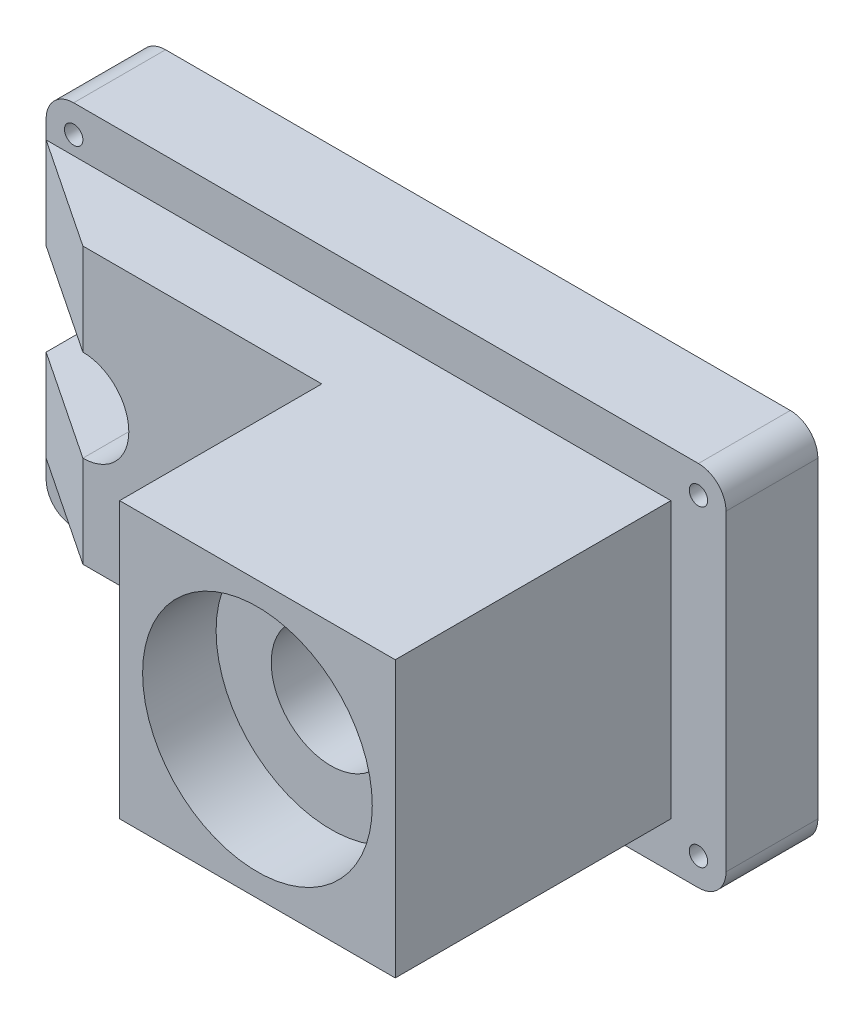
ISO-10303-21;
HEADER;
FILE_DESCRIPTION(('STEP AP214'),'2;1');
FILE_NAME('part.step','',(''),(''),'','','');
FILE_SCHEMA(('AUTOMOTIVE_DESIGN { 1 0 10303 214 1 1 1 1 }'));
ENDSEC;
DATA;
#1=APPLICATION_CONTEXT('core data for automotive mechanical design processes');
#2=APPLICATION_PROTOCOL_DEFINITION('international standard','automotive_design',2000,#1);
#3=PRODUCT_CONTEXT('',#1,'mechanical');
#4=PRODUCT('Part','Part','',(#3));
#5=PRODUCT_RELATED_PRODUCT_CATEGORY('part','',(#4));
#6=PRODUCT_DEFINITION_FORMATION('','',#4);
#7=PRODUCT_DEFINITION_CONTEXT('part definition',#1,'design');
#8=PRODUCT_DEFINITION('design','',#6,#7);
#9=PRODUCT_DEFINITION_SHAPE('','',#8);
#10=(LENGTH_UNIT() NAMED_UNIT(*) SI_UNIT(.MILLI.,.METRE.));
#11=(NAMED_UNIT(*) PLANE_ANGLE_UNIT() SI_UNIT($,.RADIAN.));
#12=(NAMED_UNIT(*) SI_UNIT($,.STERADIAN.) SOLID_ANGLE_UNIT());
#13=UNCERTAINTY_MEASURE_WITH_UNIT(LENGTH_MEASURE(1.E-05),#10,'distance_accuracy_value','');
#14=(GEOMETRIC_REPRESENTATION_CONTEXT(3) GLOBAL_UNCERTAINTY_ASSIGNED_CONTEXT((#13)) GLOBAL_UNIT_ASSIGNED_CONTEXT((#10,
#11,#12)) REPRESENTATION_CONTEXT('',''));
#15=CARTESIAN_POINT('',(0.,0.,0.));
#16=DIRECTION('',(0.,0.,1.));
#17=DIRECTION('',(1.,0.,0.));
#18=AXIS2_PLACEMENT_3D('',#15,#16,#17);
#19=CARTESIAN_POINT('',(3.,37.,10.));
#20=DIRECTION('',(0.,0.,1.));
#21=DIRECTION('',(1.,0.,0.));
#22=AXIS2_PLACEMENT_3D('',#19,#20,#21);
#23=PLANE('',#22);
#24=CARTESIAN_POINT('',(3.,3.,10.));
#25=DIRECTION('',(0.,0.,1.));
#26=DIRECTION('',(1.,0.,0.));
#27=AXIS2_PLACEMENT_3D('',#24,#25,#26);
#28=CIRCLE('',#27,1.);
#29=CARTESIAN_POINT('',(4.,3.,10.));
#30=VERTEX_POINT('',#29);
#31=EDGE_CURVE('E352',#30,#30,#28,.T.);
#32=ORIENTED_EDGE('',*,*,#31,.F.);
#33=EDGE_LOOP('',(#32));
#34=FACE_BOUND('',#33,.T.);
#35=CARTESIAN_POINT('',(71.,3.,10.));
#36=DIRECTION('',(0.,0.,1.));
#37=DIRECTION('',(1.,0.,0.));
#38=AXIS2_PLACEMENT_3D('',#35,#36,#37);
#39=CIRCLE('',#38,0.999999999999998);
#40=CARTESIAN_POINT('',(72.,3.,10.));
#41=VERTEX_POINT('',#40);
#42=EDGE_CURVE('E356',#41,#41,#39,.T.);
#43=ORIENTED_EDGE('',*,*,#42,.F.);
#44=EDGE_LOOP('',(#43));
#45=FACE_BOUND('',#44,.T.);
#46=CARTESIAN_POINT('',(71.,37.,10.));
#47=DIRECTION('',(0.,0.,1.));
#48=DIRECTION('',(1.,0.,0.));
#49=AXIS2_PLACEMENT_3D('',#46,#47,#48);
#50=CIRCLE('',#49,0.999999999999998);
#51=CARTESIAN_POINT('',(72.,37.,10.));
#52=VERTEX_POINT('',#51);
#53=EDGE_CURVE('E364',#52,#52,#50,.T.);
#54=ORIENTED_EDGE('',*,*,#53,.F.);
#55=EDGE_LOOP('',(#54));
#56=FACE_BOUND('',#55,.T.);
#57=CARTESIAN_POINT('',(3.,37.,10.));
#58=DIRECTION('',(0.,0.,1.));
#59=DIRECTION('',(1.,0.,0.));
#60=AXIS2_PLACEMENT_3D('',#57,#58,#59);
#61=CIRCLE('',#60,0.999999999999998);
#62=CARTESIAN_POINT('',(4.,37.,10.));
#63=VERTEX_POINT('',#62);
#64=EDGE_CURVE('E342',#63,#63,#61,.T.);
#65=ORIENTED_EDGE('',*,*,#64,.F.);
#66=EDGE_LOOP('',(#65));
#67=FACE_BOUND('',#66,.T.);
#68=DIRECTION('',(0.,-1.,0.));
#69=VECTOR('',#68,1.);
#70=CARTESIAN_POINT('',(0.,37.,10.));
#71=LINE('',#70,#69);
#72=CARTESIAN_POINT('',(0.,37.,10.));
#73=VERTEX_POINT('',#72);
#74=CARTESIAN_POINT('',(0.,35.,10.));
#75=VERTEX_POINT('',#74);
#76=EDGE_CURVE('E247',#73,#75,#71,.T.);
#77=ORIENTED_EDGE('',*,*,#76,.T.);
#78=DIRECTION('',(-1.,0.,0.));
#79=VECTOR('',#78,1.);
#80=CARTESIAN_POINT('',(68.,35.,10.));
#81=LINE('',#80,#79);
#82=CARTESIAN_POINT('',(68.,35.,10.));
#83=VERTEX_POINT('',#82);
#84=EDGE_CURVE('E58',#83,#75,#81,.T.);
#85=ORIENTED_EDGE('',*,*,#84,.F.);
#86=DIRECTION('',(0.,1.,0.));
#87=VECTOR('',#86,1.);
#88=CARTESIAN_POINT('',(68.,35.,10.));
#89=LINE('',#88,#87);
#90=CARTESIAN_POINT('',(68.,4.99999999999999,10.));
#91=VERTEX_POINT('',#90);
#92=EDGE_CURVE('E216',#91,#83,#89,.T.);
#93=ORIENTED_EDGE('',*,*,#92,.F.);
#94=DIRECTION('',(1.,0.,0.));
#95=VECTOR('',#94,1.);
#96=CARTESIAN_POINT('',(68.,4.99999999999999,10.));
#97=LINE('',#96,#95);
#98=CARTESIAN_POINT('',(0.,4.99999999999998,10.));
#99=VERTEX_POINT('',#98);
#100=EDGE_CURVE('E69',#99,#91,#97,.T.);
#101=ORIENTED_EDGE('',*,*,#100,.F.);
#102=DIRECTION('',(0.,-1.,0.));
#103=VECTOR('',#102,1.);
#104=CARTESIAN_POINT('',(0.,15.,10.));
#105=LINE('',#104,#103);
#106=CARTESIAN_POINT('',(0.,3.,10.));
#107=VERTEX_POINT('',#106);
#108=EDGE_CURVE('E255',#99,#107,#105,.T.);
#109=ORIENTED_EDGE('',*,*,#108,.T.);
#110=CARTESIAN_POINT('',(3.,3.,10.));
#111=DIRECTION('',(0.,0.,1.));
#112=DIRECTION('',(1.,0.,0.));
#113=AXIS2_PLACEMENT_3D('',#110,#111,#112);
#114=CIRCLE('',#113,3.);
#115=CARTESIAN_POINT('',(3.,0.,10.));
#116=VERTEX_POINT('',#115);
#117=EDGE_CURVE('E253',#107,#116,#114,.T.);
#118=ORIENTED_EDGE('',*,*,#117,.T.);
#119=DIRECTION('',(1.,0.,0.));
#120=VECTOR('',#119,1.);
#121=CARTESIAN_POINT('',(3.,0.,10.));
#122=LINE('',#121,#120);
#123=CARTESIAN_POINT('',(71.,0.,10.));
#124=VERTEX_POINT('',#123);
#125=EDGE_CURVE('E256',#116,#124,#122,.T.);
#126=ORIENTED_EDGE('',*,*,#125,.T.);
#127=CARTESIAN_POINT('',(71.,3.,10.));
#128=DIRECTION('',(0.,0.,1.));
#129=DIRECTION('',(1.,0.,0.));
#130=AXIS2_PLACEMENT_3D('',#127,#128,#129);
#131=CIRCLE('',#130,3.);
#132=CARTESIAN_POINT('',(74.,3.,10.));
#133=VERTEX_POINT('',#132);
#134=EDGE_CURVE('E258',#124,#133,#131,.T.);
#135=ORIENTED_EDGE('',*,*,#134,.T.);
#136=DIRECTION('',(0.,1.,0.));
#137=VECTOR('',#136,1.);
#138=CARTESIAN_POINT('',(74.,37.,10.));
#139=LINE('',#138,#137);
#140=CARTESIAN_POINT('',(74.,37.,10.));
#141=VERTEX_POINT('',#140);
#142=EDGE_CURVE('E262',#133,#141,#139,.T.);
#143=ORIENTED_EDGE('',*,*,#142,.T.);
#144=CARTESIAN_POINT('',(71.,37.,10.));
#145=DIRECTION('',(0.,0.,1.));
#146=DIRECTION('',(1.,0.,0.));
#147=AXIS2_PLACEMENT_3D('',#144,#145,#146);
#148=CIRCLE('',#147,3.00000000000001);
#149=CARTESIAN_POINT('',(71.,40.,10.));
#150=VERTEX_POINT('',#149);
#151=EDGE_CURVE('E264',#141,#150,#148,.T.);
#152=ORIENTED_EDGE('',*,*,#151,.T.);
#153=DIRECTION('',(-1.,0.,0.));
#154=VECTOR('',#153,1.);
#155=CARTESIAN_POINT('',(3.,40.,10.));
#156=LINE('',#155,#154);
#157=CARTESIAN_POINT('',(3.,40.,10.));
#158=VERTEX_POINT('',#157);
#159=EDGE_CURVE('E263',#150,#158,#156,.T.);
#160=ORIENTED_EDGE('',*,*,#159,.T.);
#161=CARTESIAN_POINT('',(3.,37.,10.));
#162=DIRECTION('',(0.,0.,1.));
#163=DIRECTION('',(1.,0.,0.));
#164=AXIS2_PLACEMENT_3D('',#161,#162,#163);
#165=CIRCLE('',#164,3.);
#166=EDGE_CURVE('E244',#158,#73,#165,.T.);
#167=ORIENTED_EDGE('',*,*,#166,.T.);
#168=EDGE_LOOP('',(#77,#85,#93,#101,#109,#118,#126,#135,#143,#152,#160,#167));
#169=FACE_BOUND('',#168,.T.);
#170=ADVANCED_FACE('F44',(#34,#45,#56,#67,#169),#23,.T.);
#171=CARTESIAN_POINT('',(38.,35.,40.));
#172=DIRECTION('',(1.,0.,0.));
#173=DIRECTION('',(0.,0.,-1.));
#174=AXIS2_PLACEMENT_3D('',#171,#172,#173);
#175=PLANE('',#174);
#176=DIRECTION('',(0.,1.,0.));
#177=VECTOR('',#176,1.);
#178=CARTESIAN_POINT('',(38.,35.,18.));
#179=LINE('',#178,#177);
#180=CARTESIAN_POINT('',(38.,4.99999999999999,18.));
#181=VERTEX_POINT('',#180);
#182=CARTESIAN_POINT('',(38.,35.,18.));
#183=VERTEX_POINT('',#182);
#184=EDGE_CURVE('E193',#181,#183,#179,.T.);
#185=ORIENTED_EDGE('',*,*,#184,.F.);
#186=DIRECTION('',(0.,0.,-1.));
#187=VECTOR('',#186,1.);
#188=CARTESIAN_POINT('',(38.,4.99999999999999,40.));
#189=LINE('',#188,#187);
#190=CARTESIAN_POINT('',(38.,4.99999999999999,40.));
#191=VERTEX_POINT('',#190);
#192=EDGE_CURVE('E236',#191,#181,#189,.T.);
#193=ORIENTED_EDGE('',*,*,#192,.F.);
#194=DIRECTION('',(0.,-1.,0.));
#195=VECTOR('',#194,1.);
#196=CARTESIAN_POINT('',(38.,35.,40.));
#197=LINE('',#196,#195);
#198=CARTESIAN_POINT('',(38.,35.,40.));
#199=VERTEX_POINT('',#198);
#200=EDGE_CURVE('E223',#199,#191,#197,.T.);
#201=ORIENTED_EDGE('',*,*,#200,.F.);
#202=DIRECTION('',(0.,0.,-1.));
#203=VECTOR('',#202,1.);
#204=CARTESIAN_POINT('',(38.,35.,40.));
#205=LINE('',#204,#203);
#206=EDGE_CURVE('E237',#199,#183,#205,.T.);
#207=ORIENTED_EDGE('',*,*,#206,.T.);
#208=EDGE_LOOP('',(#185,#193,#201,#207));
#209=FACE_BOUND('',#208,.T.);
#210=ADVANCED_FACE('F331',(#209),#175,.F.);
#211=CARTESIAN_POINT('',(3.,37.,10.));
#212=DIRECTION('',(0.,0.,-1.));
#213=DIRECTION('',(-1.,0.,0.));
#214=AXIS2_PLACEMENT_3D('',#211,#212,#213);
#215=CYLINDRICAL_SURFACE('',#214,3.);
#216=CARTESIAN_POINT('',(3.,37.,0.));
#217=DIRECTION('',(0.,0.,1.));
#218=DIRECTION('',(1.,0.,0.));
#219=AXIS2_PLACEMENT_3D('',#216,#217,#218);
#220=CIRCLE('',#219,3.);
#221=CARTESIAN_POINT('',(3.,40.,0.));
#222=VERTEX_POINT('',#221);
#223=CARTESIAN_POINT('',(0.,37.,0.));
#224=VERTEX_POINT('',#223);
#225=EDGE_CURVE('E242',#222,#224,#220,.T.);
#226=ORIENTED_EDGE('',*,*,#225,.T.);
#227=DIRECTION('',(0.,0.,-1.));
#228=VECTOR('',#227,1.);
#229=CARTESIAN_POINT('',(0.,37.,10.));
#230=LINE('',#229,#228);
#231=EDGE_CURVE('E11',#73,#224,#230,.T.);
#232=ORIENTED_EDGE('',*,*,#231,.F.);
#233=ORIENTED_EDGE('',*,*,#166,.F.);
#234=DIRECTION('',(0.,0.,-1.));
#235=VECTOR('',#234,1.);
#236=CARTESIAN_POINT('',(3.,40.,10.));
#237=LINE('',#236,#235);
#238=EDGE_CURVE('E270',#158,#222,#237,.T.);
#239=ORIENTED_EDGE('',*,*,#238,.T.);
#240=EDGE_LOOP('',(#226,#232,#233,#239));
#241=FACE_BOUND('',#240,.T.);
#242=ADVANCED_FACE('F50',(#241),#215,.T.);
#243=CARTESIAN_POINT('',(0.,37.,10.));
#244=DIRECTION('',(1.,0.,0.));
#245=DIRECTION('',(0.,0.,-1.));
#246=AXIS2_PLACEMENT_3D('',#243,#244,#245);
#247=PLANE('',#246);
#248=DIRECTION('',(0.,-1.,0.));
#249=VECTOR('',#248,1.);
#250=CARTESIAN_POINT('',(0.,37.,0.));
#251=LINE('',#250,#249);
#252=CARTESIAN_POINT('',(0.,25.,0.));
#253=VERTEX_POINT('',#252);
#254=EDGE_CURVE('E268',#224,#253,#251,.T.);
#255=ORIENTED_EDGE('',*,*,#254,.T.);
#256=DIRECTION('',(0.,0.,-1.));
#257=VECTOR('',#256,1.);
#258=CARTESIAN_POINT('',(0.,25.,10.));
#259=LINE('',#258,#257);
#260=CARTESIAN_POINT('',(0.,25.,10.));
#261=VERTEX_POINT('',#260);
#262=EDGE_CURVE('E52',#261,#253,#259,.T.);
#263=ORIENTED_EDGE('',*,*,#262,.F.);
#264=DIRECTION('',(0.,1.,0.));
#265=VECTOR('',#264,1.);
#266=CARTESIAN_POINT('',(0.,25.,10.));
#267=LINE('',#266,#265);
#268=EDGE_CURVE('E209',#261,#75,#267,.T.);
#269=ORIENTED_EDGE('',*,*,#268,.T.);
#270=ORIENTED_EDGE('',*,*,#76,.F.);
#271=ORIENTED_EDGE('',*,*,#231,.T.);
#272=EDGE_LOOP('',(#255,#263,#269,#270,#271));
#273=FACE_BOUND('',#272,.T.);
#274=ADVANCED_FACE('F415',(#273),#247,.F.);
#275=CARTESIAN_POINT('',(12.,25.,10.));
#276=DIRECTION('',(0.,1.,0.));
#277=DIRECTION('',(0.,0.,1.));
#278=AXIS2_PLACEMENT_3D('',#275,#276,#277);
#279=PLANE('',#278);
#280=DIRECTION('',(1.,0.,0.));
#281=VECTOR('',#280,1.);
#282=CARTESIAN_POINT('',(12.,25.,0.));
#283=LINE('',#282,#281);
#284=CARTESIAN_POINT('',(12.,25.,0.));
#285=VERTEX_POINT('',#284);
#286=EDGE_CURVE('E275',#253,#285,#283,.T.);
#287=ORIENTED_EDGE('',*,*,#286,.T.);
#288=DIRECTION('',(0.,0.,-1.));
#289=VECTOR('',#288,1.);
#290=CARTESIAN_POINT('',(12.,25.,10.));
#291=LINE('',#290,#289);
#292=CARTESIAN_POINT('',(12.,25.,18.));
#293=VERTEX_POINT('',#292);
#294=EDGE_CURVE('E185',#293,#285,#291,.T.);
#295=ORIENTED_EDGE('',*,*,#294,.F.);
#296=DIRECTION('',(0.832050294337844,0.,0.554700196225229));
#297=VECTOR('',#296,1.);
#298=CARTESIAN_POINT('',(0.,25.,10.));
#299=LINE('',#298,#297);
#300=EDGE_CURVE('E317',#261,#293,#299,.T.);
#301=ORIENTED_EDGE('',*,*,#300,.F.);
#302=ORIENTED_EDGE('',*,*,#262,.T.);
#303=EDGE_LOOP('',(#287,#295,#301,#302));
#304=FACE_BOUND('',#303,.T.);
#305=ADVANCED_FACE('F314',(#304),#279,.F.);
#306=CARTESIAN_POINT('',(12.,20.,10.));
#307=DIRECTION('',(0.,0.,-1.));
#308=DIRECTION('',(-1.,0.,0.));
#309=AXIS2_PLACEMENT_3D('',#306,#307,#308);
#310=CYLINDRICAL_SURFACE('',#309,5.);
#311=CARTESIAN_POINT('',(12.,20.,0.));
#312=DIRECTION('',(0.,0.,-1.));
#313=DIRECTION('',(1.,0.,0.));
#314=AXIS2_PLACEMENT_3D('',#311,#312,#313);
#315=CIRCLE('',#314,5.);
#316=CARTESIAN_POINT('',(12.,15.,0.));
#317=VERTEX_POINT('',#316);
#318=EDGE_CURVE('E178',#285,#317,#315,.T.);
#319=ORIENTED_EDGE('',*,*,#318,.T.);
#320=DIRECTION('',(0.,0.,-1.));
#321=VECTOR('',#320,1.);
#322=CARTESIAN_POINT('',(12.,15.,10.));
#323=LINE('',#322,#321);
#324=CARTESIAN_POINT('',(12.,15.,18.));
#325=VERTEX_POINT('',#324);
#326=EDGE_CURVE('E171',#325,#317,#323,.T.);
#327=ORIENTED_EDGE('',*,*,#326,.F.);
#328=CARTESIAN_POINT('',(12.,20.,18.));
#329=DIRECTION('',(0.,0.,-1.));
#330=DIRECTION('',(-1.,0.,0.));
#331=AXIS2_PLACEMENT_3D('',#328,#329,#330);
#332=CIRCLE('',#331,5.);
#333=EDGE_CURVE('E174',#293,#325,#332,.T.);
#334=ORIENTED_EDGE('',*,*,#333,.F.);
#335=ORIENTED_EDGE('',*,*,#294,.T.);
#336=EDGE_LOOP('',(#319,#327,#334,#335));
#337=FACE_BOUND('',#336,.T.);
#338=ADVANCED_FACE('F173',(#337),#310,.F.);
#339=CARTESIAN_POINT('',(12.,15.,10.));
#340=DIRECTION('',(0.,-1.,0.));
#341=DIRECTION('',(0.,0.,-1.));
#342=AXIS2_PLACEMENT_3D('',#339,#340,#341);
#343=PLANE('',#342);
#344=DIRECTION('',(-1.,0.,0.));
#345=VECTOR('',#344,1.);
#346=CARTESIAN_POINT('',(12.,15.,0.));
#347=LINE('',#346,#345);
#348=CARTESIAN_POINT('',(0.,15.,0.));
#349=VERTEX_POINT('',#348);
#350=EDGE_CURVE('E273',#317,#349,#347,.T.);
#351=ORIENTED_EDGE('',*,*,#350,.T.);
#352=DIRECTION('',(0.,0.,-1.));
#353=VECTOR('',#352,1.);
#354=CARTESIAN_POINT('',(0.,15.,10.));
#355=LINE('',#354,#353);
#356=CARTESIAN_POINT('',(0.,15.,10.));
#357=VERTEX_POINT('',#356);
#358=EDGE_CURVE('E182',#357,#349,#355,.T.);
#359=ORIENTED_EDGE('',*,*,#358,.F.);
#360=DIRECTION('',(-0.832050294337844,0.,-0.554700196225229));
#361=VECTOR('',#360,1.);
#362=CARTESIAN_POINT('',(12.,15.,18.));
#363=LINE('',#362,#361);
#364=EDGE_CURVE('E192',#325,#357,#363,.T.);
#365=ORIENTED_EDGE('',*,*,#364,.F.);
#366=ORIENTED_EDGE('',*,*,#326,.T.);
#367=EDGE_LOOP('',(#351,#359,#365,#366));
#368=FACE_BOUND('',#367,.T.);
#369=ADVANCED_FACE('F203',(#368),#343,.F.);
#370=CARTESIAN_POINT('',(0.,15.,10.));
#371=DIRECTION('',(1.,0.,0.));
#372=DIRECTION('',(0.,0.,-1.));
#373=AXIS2_PLACEMENT_3D('',#370,#371,#372);
#374=PLANE('',#373);
#375=DIRECTION('',(0.,-1.,0.));
#376=VECTOR('',#375,1.);
#377=CARTESIAN_POINT('',(0.,15.,0.));
#378=LINE('',#377,#376);
#379=CARTESIAN_POINT('',(0.,3.,0.));
#380=VERTEX_POINT('',#379);
#381=EDGE_CURVE('E276',#349,#380,#378,.T.);
#382=ORIENTED_EDGE('',*,*,#381,.T.);
#383=DIRECTION('',(0.,0.,-1.));
#384=VECTOR('',#383,1.);
#385=CARTESIAN_POINT('',(0.,3.,10.));
#386=LINE('',#385,#384);
#387=EDGE_CURVE('E310',#107,#380,#386,.T.);
#388=ORIENTED_EDGE('',*,*,#387,.F.);
#389=ORIENTED_EDGE('',*,*,#108,.F.);
#390=EDGE_CURVE('E254',#357,#99,#105,.T.);
#391=ORIENTED_EDGE('',*,*,#390,.F.);
#392=ORIENTED_EDGE('',*,*,#358,.T.);
#393=EDGE_LOOP('',(#382,#388,#389,#391,#392));
#394=FACE_BOUND('',#393,.T.);
#395=ADVANCED_FACE('F322',(#394),#374,.F.);
#396=CARTESIAN_POINT('',(3.,3.,10.));
#397=DIRECTION('',(0.,0.,-1.));
#398=DIRECTION('',(-1.,0.,0.));
#399=AXIS2_PLACEMENT_3D('',#396,#397,#398);
#400=CYLINDRICAL_SURFACE('',#399,3.);
#401=CARTESIAN_POINT('',(3.,3.,0.));
#402=DIRECTION('',(0.,0.,1.));
#403=DIRECTION('',(1.,0.,0.));
#404=AXIS2_PLACEMENT_3D('',#401,#402,#403);
#405=CIRCLE('',#404,3.);
#406=CARTESIAN_POINT('',(3.,0.,0.));
#407=VERTEX_POINT('',#406);
#408=EDGE_CURVE('E278',#380,#407,#405,.T.);
#409=ORIENTED_EDGE('',*,*,#408,.T.);
#410=DIRECTION('',(0.,0.,-1.));
#411=VECTOR('',#410,1.);
#412=CARTESIAN_POINT('',(3.,0.,10.));
#413=LINE('',#412,#411);
#414=EDGE_CURVE('E302',#116,#407,#413,.T.);
#415=ORIENTED_EDGE('',*,*,#414,.F.);
#416=ORIENTED_EDGE('',*,*,#117,.F.);
#417=ORIENTED_EDGE('',*,*,#387,.T.);
#418=EDGE_LOOP('',(#409,#415,#416,#417));
#419=FACE_BOUND('',#418,.T.);
#420=ADVANCED_FACE('F445',(#419),#400,.T.);
#421=CARTESIAN_POINT('',(3.,0.,10.));
#422=DIRECTION('',(0.,1.,0.));
#423=DIRECTION('',(0.,0.,1.));
#424=AXIS2_PLACEMENT_3D('',#421,#422,#423);
#425=PLANE('',#424);
#426=DIRECTION('',(1.,0.,0.));
#427=VECTOR('',#426,1.);
#428=CARTESIAN_POINT('',(3.,0.,0.));
#429=LINE('',#428,#427);
#430=CARTESIAN_POINT('',(71.,0.,0.));
#431=VERTEX_POINT('',#430);
#432=EDGE_CURVE('E282',#407,#431,#429,.T.);
#433=ORIENTED_EDGE('',*,*,#432,.T.);
#434=DIRECTION('',(0.,0.,-1.));
#435=VECTOR('',#434,1.);
#436=CARTESIAN_POINT('',(71.,0.,10.));
#437=LINE('',#436,#435);
#438=EDGE_CURVE('E301',#124,#431,#437,.T.);
#439=ORIENTED_EDGE('',*,*,#438,.F.);
#440=ORIENTED_EDGE('',*,*,#125,.F.);
#441=ORIENTED_EDGE('',*,*,#414,.T.);
#442=EDGE_LOOP('',(#433,#439,#440,#441));
#443=FACE_BOUND('',#442,.T.);
#444=ADVANCED_FACE('F438',(#443),#425,.F.);
#445=CARTESIAN_POINT('',(71.,3.,10.));
#446=DIRECTION('',(0.,0.,-1.));
#447=DIRECTION('',(-1.,0.,0.));
#448=AXIS2_PLACEMENT_3D('',#445,#446,#447);
#449=CYLINDRICAL_SURFACE('',#448,3.);
#450=CARTESIAN_POINT('',(71.,3.,0.));
#451=DIRECTION('',(0.,0.,1.));
#452=DIRECTION('',(1.,0.,0.));
#453=AXIS2_PLACEMENT_3D('',#450,#451,#452);
#454=CIRCLE('',#453,3.);
#455=CARTESIAN_POINT('',(74.,3.,0.));
#456=VERTEX_POINT('',#455);
#457=EDGE_CURVE('E284',#431,#456,#454,.T.);
#458=ORIENTED_EDGE('',*,*,#457,.T.);
#459=DIRECTION('',(0.,0.,-1.));
#460=VECTOR('',#459,1.);
#461=CARTESIAN_POINT('',(74.,3.,10.));
#462=LINE('',#461,#460);
#463=EDGE_CURVE('E296',#133,#456,#462,.T.);
#464=ORIENTED_EDGE('',*,*,#463,.F.);
#465=ORIENTED_EDGE('',*,*,#134,.F.);
#466=ORIENTED_EDGE('',*,*,#438,.T.);
#467=EDGE_LOOP('',(#458,#464,#465,#466));
#468=FACE_BOUND('',#467,.T.);
#469=ADVANCED_FACE('F433',(#468),#449,.T.);
#470=CARTESIAN_POINT('',(74.,37.,10.));
#471=DIRECTION('',(-1.,0.,0.));
#472=DIRECTION('',(0.,0.,1.));
#473=AXIS2_PLACEMENT_3D('',#470,#471,#472);
#474=PLANE('',#473);
#475=DIRECTION('',(0.,1.,0.));
#476=VECTOR('',#475,1.);
#477=CARTESIAN_POINT('',(74.,37.,0.));
#478=LINE('',#477,#476);
#479=CARTESIAN_POINT('',(74.,37.,0.));
#480=VERTEX_POINT('',#479);
#481=EDGE_CURVE('E283',#456,#480,#478,.T.);
#482=ORIENTED_EDGE('',*,*,#481,.T.);
#483=DIRECTION('',(0.,0.,-1.));
#484=VECTOR('',#483,1.);
#485=CARTESIAN_POINT('',(74.,37.,10.));
#486=LINE('',#485,#484);
#487=EDGE_CURVE('E294',#141,#480,#486,.T.);
#488=ORIENTED_EDGE('',*,*,#487,.F.);
#489=ORIENTED_EDGE('',*,*,#142,.F.);
#490=ORIENTED_EDGE('',*,*,#463,.T.);
#491=EDGE_LOOP('',(#482,#488,#489,#490));
#492=FACE_BOUND('',#491,.T.);
#493=ADVANCED_FACE('F426',(#492),#474,.F.);
#494=CARTESIAN_POINT('',(71.,37.,10.));
#495=DIRECTION('',(0.,0.,-1.));
#496=DIRECTION('',(-1.,0.,0.));
#497=AXIS2_PLACEMENT_3D('',#494,#495,#496);
#498=CYLINDRICAL_SURFACE('',#497,3.00000000000001);
#499=CARTESIAN_POINT('',(71.,37.,0.));
#500=DIRECTION('',(0.,0.,1.));
#501=DIRECTION('',(1.,0.,0.));
#502=AXIS2_PLACEMENT_3D('',#499,#500,#501);
#503=CIRCLE('',#502,3.00000000000001);
#504=CARTESIAN_POINT('',(71.,40.,0.));
#505=VERTEX_POINT('',#504);
#506=EDGE_CURVE('E290',#480,#505,#503,.T.);
#507=ORIENTED_EDGE('',*,*,#506,.T.);
#508=DIRECTION('',(0.,0.,-1.));
#509=VECTOR('',#508,1.);
#510=CARTESIAN_POINT('',(71.,40.,10.));
#511=LINE('',#510,#509);
#512=EDGE_CURVE('E292',#150,#505,#511,.T.);
#513=ORIENTED_EDGE('',*,*,#512,.F.);
#514=ORIENTED_EDGE('',*,*,#151,.F.);
#515=ORIENTED_EDGE('',*,*,#487,.T.);
#516=EDGE_LOOP('',(#507,#513,#514,#515));
#517=FACE_BOUND('',#516,.T.);
#518=ADVANCED_FACE('F425',(#517),#498,.T.);
#519=CARTESIAN_POINT('',(3.,40.,10.));
#520=DIRECTION('',(0.,-1.,0.));
#521=DIRECTION('',(1.,0.,0.));
#522=AXIS2_PLACEMENT_3D('',#519,#520,#521);
#523=PLANE('',#522);
#524=DIRECTION('',(-1.,0.,0.));
#525=VECTOR('',#524,1.);
#526=CARTESIAN_POINT('',(3.,40.,0.));
#527=LINE('',#526,#525);
#528=EDGE_CURVE('E248',#505,#222,#527,.T.);
#529=ORIENTED_EDGE('',*,*,#528,.T.);
#530=ORIENTED_EDGE('',*,*,#238,.F.);
#531=ORIENTED_EDGE('',*,*,#159,.F.);
#532=ORIENTED_EDGE('',*,*,#512,.T.);
#533=EDGE_LOOP('',(#529,#530,#531,#532));
#534=FACE_BOUND('',#533,.T.);
#535=ADVANCED_FACE('F416',(#534),#523,.F.);
#536=CARTESIAN_POINT('',(3.,37.,0.));
#537=DIRECTION('',(0.,0.,1.));
#538=DIRECTION('',(1.,0.,0.));
#539=AXIS2_PLACEMENT_3D('',#536,#537,#538);
#540=PLANE('',#539);
#541=CARTESIAN_POINT('',(3.,3.,0.));
#542=DIRECTION('',(0.,0.,1.));
#543=DIRECTION('',(1.,0.,0.));
#544=AXIS2_PLACEMENT_3D('',#541,#542,#543);
#545=CIRCLE('',#544,1.);
#546=CARTESIAN_POINT('',(4.,3.,0.));
#547=VERTEX_POINT('',#546);
#548=EDGE_CURVE('E351',#547,#547,#545,.T.);
#549=ORIENTED_EDGE('',*,*,#548,.T.);
#550=EDGE_LOOP('',(#549));
#551=FACE_BOUND('',#550,.T.);
#552=CARTESIAN_POINT('',(71.,3.,0.));
#553=DIRECTION('',(0.,0.,1.));
#554=DIRECTION('',(1.,0.,0.));
#555=AXIS2_PLACEMENT_3D('',#552,#553,#554);
#556=CIRCLE('',#555,0.999999999999998);
#557=CARTESIAN_POINT('',(72.,3.,0.));
#558=VERTEX_POINT('',#557);
#559=EDGE_CURVE('E363',#558,#558,#556,.T.);
#560=ORIENTED_EDGE('',*,*,#559,.T.);
#561=EDGE_LOOP('',(#560));
#562=FACE_BOUND('',#561,.T.);
#563=CARTESIAN_POINT('',(71.,37.,0.));
#564=DIRECTION('',(0.,0.,1.));
#565=DIRECTION('',(1.,0.,0.));
#566=AXIS2_PLACEMENT_3D('',#563,#564,#565);
#567=CIRCLE('',#566,0.999999999999998);
#568=CARTESIAN_POINT('',(72.,37.,0.));
#569=VERTEX_POINT('',#568);
#570=EDGE_CURVE('E349',#569,#569,#567,.T.);
#571=ORIENTED_EDGE('',*,*,#570,.T.);
#572=EDGE_LOOP('',(#571));
#573=FACE_BOUND('',#572,.T.);
#574=CARTESIAN_POINT('',(3.,37.,0.));
#575=DIRECTION('',(0.,0.,1.));
#576=DIRECTION('',(1.,0.,0.));
#577=AXIS2_PLACEMENT_3D('',#574,#575,#576);
#578=CIRCLE('',#577,0.999999999999998);
#579=CARTESIAN_POINT('',(4.,37.,0.));
#580=VERTEX_POINT('',#579);
#581=EDGE_CURVE('E345',#580,#580,#578,.T.);
#582=ORIENTED_EDGE('',*,*,#581,.T.);
#583=EDGE_LOOP('',(#582));
#584=FACE_BOUND('',#583,.T.);
#585=ORIENTED_EDGE('',*,*,#225,.F.);
#586=ORIENTED_EDGE('',*,*,#528,.F.);
#587=ORIENTED_EDGE('',*,*,#506,.F.);
#588=ORIENTED_EDGE('',*,*,#481,.F.);
#589=ORIENTED_EDGE('',*,*,#457,.F.);
#590=ORIENTED_EDGE('',*,*,#432,.F.);
#591=ORIENTED_EDGE('',*,*,#408,.F.);
#592=ORIENTED_EDGE('',*,*,#381,.F.);
#593=ORIENTED_EDGE('',*,*,#350,.F.);
#594=ORIENTED_EDGE('',*,*,#318,.F.);
#595=ORIENTED_EDGE('',*,*,#286,.F.);
#596=ORIENTED_EDGE('',*,*,#254,.F.);
#597=EDGE_LOOP('',(#585,#586,#587,#588,#589,#590,#591,#592,#593,#594,#595,#596));
#598=FACE_BOUND('',#597,.T.);
#599=ADVANCED_FACE('F324',(#551,#562,#573,#584,#598),#540,.F.);
#600=CARTESIAN_POINT('',(68.,35.,40.));
#601=DIRECTION('',(-1.,0.,0.));
#602=DIRECTION('',(0.,0.,1.));
#603=AXIS2_PLACEMENT_3D('',#600,#601,#602);
#604=PLANE('',#603);
#605=ORIENTED_EDGE('',*,*,#92,.T.);
#606=DIRECTION('',(0.,0.,-1.));
#607=VECTOR('',#606,1.);
#608=CARTESIAN_POINT('',(68.,35.,40.));
#609=LINE('',#608,#607);
#610=CARTESIAN_POINT('',(68.,35.,40.));
#611=VERTEX_POINT('',#610);
#612=EDGE_CURVE('E245',#611,#83,#609,.T.);
#613=ORIENTED_EDGE('',*,*,#612,.F.);
#614=DIRECTION('',(0.,1.,0.));
#615=VECTOR('',#614,1.);
#616=CARTESIAN_POINT('',(68.,35.,40.));
#617=LINE('',#616,#615);
#618=CARTESIAN_POINT('',(68.,4.99999999999999,40.));
#619=VERTEX_POINT('',#618);
#620=EDGE_CURVE('E218',#619,#611,#617,.T.);
#621=ORIENTED_EDGE('',*,*,#620,.F.);
#622=DIRECTION('',(0.,0.,-1.));
#623=VECTOR('',#622,1.);
#624=CARTESIAN_POINT('',(68.,4.99999999999999,40.));
#625=LINE('',#624,#623);
#626=EDGE_CURVE('E230',#619,#91,#625,.T.);
#627=ORIENTED_EDGE('',*,*,#626,.T.);
#628=EDGE_LOOP('',(#605,#613,#621,#627));
#629=FACE_BOUND('',#628,.T.);
#630=ADVANCED_FACE('F408',(#629),#604,.F.);
#631=CARTESIAN_POINT('',(68.,35.,40.));
#632=DIRECTION('',(0.,-1.,0.));
#633=DIRECTION('',(1.,0.,0.));
#634=AXIS2_PLACEMENT_3D('',#631,#632,#633);
#635=PLANE('',#634);
#636=ORIENTED_EDGE('',*,*,#84,.T.);
#637=DIRECTION('',(0.832050294337844,0.,0.554700196225229));
#638=VECTOR('',#637,1.);
#639=CARTESIAN_POINT('',(0.,35.,10.));
#640=LINE('',#639,#638);
#641=CARTESIAN_POINT('',(12.,35.,18.));
#642=VERTEX_POINT('',#641);
#643=EDGE_CURVE('E339',#75,#642,#640,.T.);
#644=ORIENTED_EDGE('',*,*,#643,.T.);
#645=DIRECTION('',(1.,0.,0.));
#646=VECTOR('',#645,1.);
#647=CARTESIAN_POINT('',(12.,35.,18.));
#648=LINE('',#647,#646);
#649=EDGE_CURVE('E204',#642,#183,#648,.T.);
#650=ORIENTED_EDGE('',*,*,#649,.T.);
#651=ORIENTED_EDGE('',*,*,#206,.F.);
#652=DIRECTION('',(-1.,0.,0.));
#653=VECTOR('',#652,1.);
#654=CARTESIAN_POINT('',(68.,35.,40.));
#655=LINE('',#654,#653);
#656=EDGE_CURVE('E224',#611,#199,#655,.T.);
#657=ORIENTED_EDGE('',*,*,#656,.F.);
#658=ORIENTED_EDGE('',*,*,#612,.T.);
#659=EDGE_LOOP('',(#636,#644,#650,#651,#657,#658));
#660=FACE_BOUND('',#659,.T.);
#661=ADVANCED_FACE('F340',(#660),#635,.F.);
#662=CARTESIAN_POINT('',(68.,4.99999999999999,40.));
#663=DIRECTION('',(0.,1.,0.));
#664=DIRECTION('',(-1.,0.,0.));
#665=AXIS2_PLACEMENT_3D('',#662,#663,#664);
#666=PLANE('',#665);
#667=ORIENTED_EDGE('',*,*,#100,.T.);
#668=ORIENTED_EDGE('',*,*,#626,.F.);
#669=DIRECTION('',(1.,0.,0.));
#670=VECTOR('',#669,1.);
#671=CARTESIAN_POINT('',(68.,4.99999999999999,40.));
#672=LINE('',#671,#670);
#673=EDGE_CURVE('E227',#191,#619,#672,.T.);
#674=ORIENTED_EDGE('',*,*,#673,.F.);
#675=ORIENTED_EDGE('',*,*,#192,.T.);
#676=DIRECTION('',(1.,0.,0.));
#677=VECTOR('',#676,1.);
#678=CARTESIAN_POINT('',(12.,4.99999999999999,18.));
#679=LINE('',#678,#677);
#680=CARTESIAN_POINT('',(12.,4.99999999999999,18.));
#681=VERTEX_POINT('',#680);
#682=EDGE_CURVE('E220',#681,#181,#679,.T.);
#683=ORIENTED_EDGE('',*,*,#682,.F.);
#684=DIRECTION('',(-0.832050294337844,0.,-0.554700196225229));
#685=VECTOR('',#684,1.);
#686=CARTESIAN_POINT('',(12.,4.99999999999998,18.));
#687=LINE('',#686,#685);
#688=EDGE_CURVE('E205',#681,#99,#687,.T.);
#689=ORIENTED_EDGE('',*,*,#688,.T.);
#690=EDGE_LOOP('',(#667,#668,#674,#675,#683,#689));
#691=FACE_BOUND('',#690,.T.);
#692=ADVANCED_FACE('F329',(#691),#666,.F.);
#693=CARTESIAN_POINT('',(0.,0.,40.));
#694=DIRECTION('',(0.,0.,-1.));
#695=DIRECTION('',(-1.,0.,0.));
#696=AXIS2_PLACEMENT_3D('',#693,#694,#695);
#697=PLANE('',#696);
#698=CARTESIAN_POINT('',(53.,20.,40.));
#699=DIRECTION('',(0.,0.,1.));
#700=DIRECTION('',(1.,0.,0.));
#701=AXIS2_PLACEMENT_3D('',#698,#699,#700);
#702=CIRCLE('',#701,12.5);
#703=CARTESIAN_POINT('',(65.5,20.,40.));
#704=VERTEX_POINT('',#703);
#705=EDGE_CURVE('E367',#704,#704,#702,.T.);
#706=ORIENTED_EDGE('',*,*,#705,.F.);
#707=EDGE_LOOP('',(#706));
#708=FACE_BOUND('',#707,.T.);
#709=ORIENTED_EDGE('',*,*,#620,.T.);
#710=ORIENTED_EDGE('',*,*,#656,.T.);
#711=ORIENTED_EDGE('',*,*,#200,.T.);
#712=ORIENTED_EDGE('',*,*,#673,.T.);
#713=EDGE_LOOP('',(#709,#710,#711,#712));
#714=FACE_BOUND('',#713,.T.);
#715=ADVANCED_FACE('F405',(#708,#714),#697,.F.);
#716=CARTESIAN_POINT('',(12.,35.,18.));
#717=DIRECTION('',(0.,0.,-1.));
#718=DIRECTION('',(-1.,0.,0.));
#719=AXIS2_PLACEMENT_3D('',#716,#717,#718);
#720=PLANE('',#719);
#721=DIRECTION('',(0.,1.,0.));
#722=VECTOR('',#721,1.);
#723=CARTESIAN_POINT('',(12.,35.,18.));
#724=LINE('',#723,#722);
#725=EDGE_CURVE('E191',#293,#642,#724,.T.);
#726=ORIENTED_EDGE('',*,*,#725,.F.);
#727=ORIENTED_EDGE('',*,*,#333,.T.);
#728=EDGE_CURVE('E186',#681,#325,#724,.T.);
#729=ORIENTED_EDGE('',*,*,#728,.F.);
#730=ORIENTED_EDGE('',*,*,#682,.T.);
#731=ORIENTED_EDGE('',*,*,#184,.T.);
#732=ORIENTED_EDGE('',*,*,#649,.F.);
#733=EDGE_LOOP('',(#726,#727,#729,#730,#731,#732));
#734=FACE_BOUND('',#733,.T.);
#735=ADVANCED_FACE('F189',(#734),#720,.F.);
#736=CARTESIAN_POINT('',(12.,15.,18.));
#737=DIRECTION('',(-0.554700196225229,0.,0.832050294337844));
#738=DIRECTION('',(0.832050294337844,0.,0.554700196225229));
#739=AXIS2_PLACEMENT_3D('',#736,#737,#738);
#740=PLANE('',#739);
#741=ORIENTED_EDGE('',*,*,#688,.F.);
#742=ORIENTED_EDGE('',*,*,#728,.T.);
#743=ORIENTED_EDGE('',*,*,#364,.T.);
#744=ORIENTED_EDGE('',*,*,#390,.T.);
#745=EDGE_LOOP('',(#741,#742,#743,#744));
#746=FACE_BOUND('',#745,.T.);
#747=ADVANCED_FACE('F196',(#746),#740,.T.);
#748=CARTESIAN_POINT('',(0.,25.,10.));
#749=DIRECTION('',(-0.554700196225229,0.,0.832050294337844));
#750=DIRECTION('',(0.832050294337844,0.,0.554700196225229));
#751=AXIS2_PLACEMENT_3D('',#748,#749,#750);
#752=PLANE('',#751);
#753=ORIENTED_EDGE('',*,*,#643,.F.);
#754=ORIENTED_EDGE('',*,*,#268,.F.);
#755=ORIENTED_EDGE('',*,*,#300,.T.);
#756=ORIENTED_EDGE('',*,*,#725,.T.);
#757=EDGE_LOOP('',(#753,#754,#755,#756));
#758=FACE_BOUND('',#757,.T.);
#759=ADVANCED_FACE('F344',(#758),#752,.T.);
#760=CARTESIAN_POINT('',(3.,37.,0.));
#761=DIRECTION('',(0.,0.,1.));
#762=DIRECTION('',(1.,0.,0.));
#763=AXIS2_PLACEMENT_3D('',#760,#761,#762);
#764=CYLINDRICAL_SURFACE('',#763,0.999999999999998);
#765=ORIENTED_EDGE('',*,*,#581,.F.);
#766=EDGE_LOOP('',(#765));
#767=FACE_BOUND('',#766,.T.);
#768=ORIENTED_EDGE('',*,*,#64,.T.);
#769=EDGE_LOOP('',(#768));
#770=FACE_BOUND('',#769,.T.);
#771=ADVANCED_FACE('F584',(#767,#770),#764,.F.);
#772=CARTESIAN_POINT('',(71.,37.,0.));
#773=DIRECTION('',(0.,0.,1.));
#774=DIRECTION('',(1.,0.,0.));
#775=AXIS2_PLACEMENT_3D('',#772,#773,#774);
#776=CYLINDRICAL_SURFACE('',#775,0.999999999999998);
#777=ORIENTED_EDGE('',*,*,#570,.F.);
#778=EDGE_LOOP('',(#777));
#779=FACE_BOUND('',#778,.T.);
#780=ORIENTED_EDGE('',*,*,#53,.T.);
#781=EDGE_LOOP('',(#780));
#782=FACE_BOUND('',#781,.T.);
#783=ADVANCED_FACE('F598',(#779,#782),#776,.F.);
#784=CARTESIAN_POINT('',(71.,3.,0.));
#785=DIRECTION('',(0.,0.,1.));
#786=DIRECTION('',(1.,0.,0.));
#787=AXIS2_PLACEMENT_3D('',#784,#785,#786);
#788=CYLINDRICAL_SURFACE('',#787,0.999999999999998);
#789=ORIENTED_EDGE('',*,*,#559,.F.);
#790=EDGE_LOOP('',(#789));
#791=FACE_BOUND('',#790,.T.);
#792=ORIENTED_EDGE('',*,*,#42,.T.);
#793=EDGE_LOOP('',(#792));
#794=FACE_BOUND('',#793,.T.);
#795=ADVANCED_FACE('F614',(#791,#794),#788,.F.);
#796=CARTESIAN_POINT('',(3.,3.,0.));
#797=DIRECTION('',(0.,0.,1.));
#798=DIRECTION('',(1.,0.,0.));
#799=AXIS2_PLACEMENT_3D('',#796,#797,#798);
#800=CYLINDRICAL_SURFACE('',#799,1.);
#801=ORIENTED_EDGE('',*,*,#548,.F.);
#802=EDGE_LOOP('',(#801));
#803=FACE_BOUND('',#802,.T.);
#804=ORIENTED_EDGE('',*,*,#31,.T.);
#805=EDGE_LOOP('',(#804));
#806=FACE_BOUND('',#805,.T.);
#807=ADVANCED_FACE('F399',(#803,#806),#800,.F.);
#808=CARTESIAN_POINT('',(53.,20.,32.));
#809=DIRECTION('',(0.,0.,1.));
#810=DIRECTION('',(1.,0.,0.));
#811=AXIS2_PLACEMENT_3D('',#808,#809,#810);
#812=CYLINDRICAL_SURFACE('',#811,12.5);
#813=CARTESIAN_POINT('',(53.,20.,32.));
#814=DIRECTION('',(0.,0.,1.));
#815=DIRECTION('',(1.,0.,0.));
#816=AXIS2_PLACEMENT_3D('',#813,#814,#815);
#817=CIRCLE('',#816,12.5);
#818=CARTESIAN_POINT('',(65.5,20.,32.));
#819=VERTEX_POINT('',#818);
#820=EDGE_CURVE('E353',#819,#819,#817,.T.);
#821=ORIENTED_EDGE('',*,*,#820,.F.);
#822=EDGE_LOOP('',(#821));
#823=FACE_BOUND('',#822,.T.);
#824=ORIENTED_EDGE('',*,*,#705,.T.);
#825=EDGE_LOOP('',(#824));
#826=FACE_BOUND('',#825,.T.);
#827=ADVANCED_FACE('F395',(#823,#826),#812,.F.);
#828=CARTESIAN_POINT('',(53.,20.,32.));
#829=DIRECTION('',(0.,0.,1.));
#830=DIRECTION('',(1.,0.,0.));
#831=AXIS2_PLACEMENT_3D('',#828,#829,#830);
#832=PLANE('',#831);
#833=CARTESIAN_POINT('',(53.,20.,32.));
#834=DIRECTION('',(0.,0.,1.));
#835=DIRECTION('',(1.,0.,0.));
#836=AXIS2_PLACEMENT_3D('',#833,#834,#835);
#837=CIRCLE('',#836,6.5);
#838=CARTESIAN_POINT('',(59.5,20.,32.));
#839=VERTEX_POINT('',#838);
#840=EDGE_CURVE('E374',#839,#839,#837,.T.);
#841=ORIENTED_EDGE('',*,*,#840,.F.);
#842=EDGE_LOOP('',(#841));
#843=FACE_BOUND('',#842,.T.);
#844=ORIENTED_EDGE('',*,*,#820,.T.);
#845=EDGE_LOOP('',(#844));
#846=FACE_BOUND('',#845,.T.);
#847=ADVANCED_FACE('F389',(#843,#846),#832,.T.);
#848=CARTESIAN_POINT('',(53.,20.,24.));
#849=DIRECTION('',(0.,0.,1.));
#850=DIRECTION('',(1.,0.,0.));
#851=AXIS2_PLACEMENT_3D('',#848,#849,#850);
#852=CYLINDRICAL_SURFACE('',#851,6.5);
#853=CARTESIAN_POINT('',(53.,20.,24.));
#854=DIRECTION('',(0.,0.,1.));
#855=DIRECTION('',(1.,0.,0.));
#856=AXIS2_PLACEMENT_3D('',#853,#854,#855);
#857=CIRCLE('',#856,6.5);
#858=CARTESIAN_POINT('',(59.5,20.,24.));
#859=VERTEX_POINT('',#858);
#860=EDGE_CURVE('E375',#859,#859,#857,.T.);
#861=ORIENTED_EDGE('',*,*,#860,.F.);
#862=EDGE_LOOP('',(#861));
#863=FACE_BOUND('',#862,.T.);
#864=ORIENTED_EDGE('',*,*,#840,.T.);
#865=EDGE_LOOP('',(#864));
#866=FACE_BOUND('',#865,.T.);
#867=ADVANCED_FACE('F384',(#863,#866),#852,.F.);
#868=CARTESIAN_POINT('',(53.,20.,24.));
#869=DIRECTION('',(0.,0.,1.));
#870=DIRECTION('',(1.,0.,0.));
#871=AXIS2_PLACEMENT_3D('',#868,#869,#870);
#872=PLANE('',#871);
#873=ORIENTED_EDGE('',*,*,#860,.T.);
#874=EDGE_LOOP('',(#873));
#875=FACE_BOUND('',#874,.T.);
#876=ADVANCED_FACE('F382',(#875),#872,.T.);
#877=CLOSED_SHELL('',(#170,#210,#242,#274,#305,#338,#369,#395,#420,#444,#469,#493,#518,#535,
#599,#630,#661,#692,#715,#735,#747,#759,#771,#783,#795,#807,#827,#847,#867,#876));
#878=MANIFOLD_SOLID_BREP('B2',#877);
#879=ADVANCED_BREP_SHAPE_REPRESENTATION('',(#18,#878),#14);
#880=SHAPE_DEFINITION_REPRESENTATION(#9,#879);
ENDSEC;
END-ISO-10303-21;
